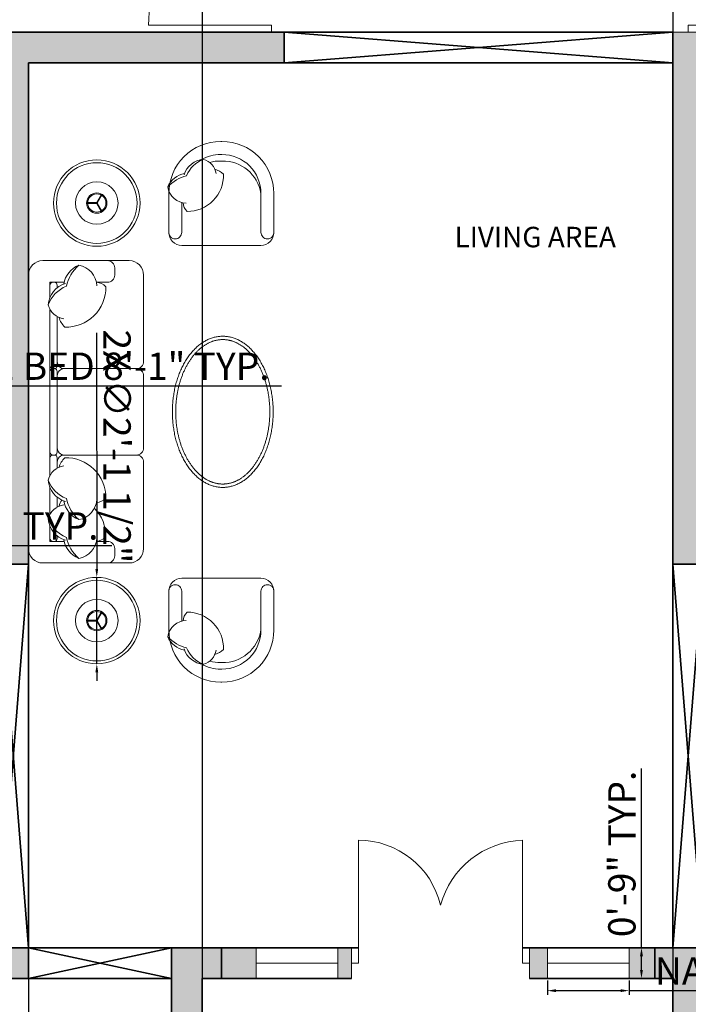
# Model space of a CAD drawing. Units: inches. Extents: x 2257 to 3678, y 834 to 1975.
# Tile 3 of 16: x 2500 to 2696, y 1155 to 1444. Entities that reach past the tile are written whole.
import ezdxf

# ---------------------------------------------------------------- set-up
doc = ezdxf.new("R2010")
doc.units = ezdxf.units.IN
for name, color, linetype, lineweight in [('A-ANNO-DIMS', 2, 'Continuous', 18), ('A-AREA-IDEN', 7, 'Continuous', 18), ('A-DOOR', 3, 'Continuous', 18), ('A-FURN', 8, 'Continuous', 18), ('A-GLAZ', 4, 'Continuous', 18), ('A-WALL', 7, 'Continuous', 35)]:
    doc.layers.add(name, color=color, linetype=linetype, lineweight=lineweight)
doc.layers.add('A-WALL-PATT', color=251, linetype='Continuous', lineweight=13, true_color=0x636466)
doc.styles.get("Standard").update_dxf_attribs({"font": 'arial.ttf'})
doc.dimstyles.new('ISO-25', dxfattribs={"dimtxt": 8, "dimasz": 2.5, "dimexe": 1.25, "dimexo": 0.625, "dimtad": 1, "dimdec": 0, "dimlunit": 3, "dimtxsty": 'Standard', "dimcen": 2.5, "dimadec": 0, "dimazin": 0, "dimtfac": 1, "dimtdec": 0, "dimtmove": 0, "dimatfit": 3, "dimfxl": 1, "dimarcsym": 0})

# ---------------------------------------------------------------- blocks, each defined once
blk = doc.blocks.new('TABLE-END-ROUND')
at = {"ltscale": 0.03}
for p, q in [((12.55, 12.73), (14.04, 15.31)), ((12.78, 12.6), (14.27, 15.18)), ((12.67, 12.8), (9.69, 12.8)), ((12.67, 12.53), (9.69, 12.53)), ((12.55, 12.6), (14.04, 10.02)), ((12.78, 12.73), (14.27, 10.15))]:
    blk.add_line(p, q, dxfattribs=at)
for radius in [12.67, 6.23, 2.98, 2.67]:
    blk.add_circle((12.67, 12.67), radius, dxfattribs=at)
blk.add_circle((12.67, 12.67), 11.82)
blk = doc.blocks.new('WIN-24')
for p, q in [((0, 9), (0, 0)), ((24, 4.5), (24, 9)), ((24, 9), (24, 0)), ((0, 0), (0, 4.5)), ((0, 4.5), (24, 4.5))]:
    blk.add_line(p, q)
blk = doc.blocks.new('DOOR-BEDROOM-REAR')
for p, q in [((36, 45), (36, 43)), ((36, 2), (0, 2)), ((36, 0), (36, 2))]:
    blk.add_line(p, q)
blk.add_arc((41.35, 2), 41.35, 97.4306, 180)
blk = doc.blocks.new('DOOR-KITCHEN')
for p, q in [((0, 45), (9, 45)), ((4.5, 45), (4.5, 43)), ((9, 45), (4.5, 45)), ((4.5, 0), (4.5, 2)), ((4.5, 2), (40.5, 2)), ((9, 0), (0, 0))]:
    blk.add_line(p, q)
blk.add_arc((4.5, 6.7), 36.3, 352.5694, 90)
blk = doc.blocks.new('DOOR-LOBBY-PAIR')
for p, q in [((2, 4.5), (2, 40.5)), ((50.14, 4.5), (50.14, 40.5)), ((0, 0), (0, 9)), ((0, 9), (0, 4.5)), ((52.14, 9), (52.14, 0)), ((0, 4.5), (2, 4.5)), ((52.14, 4.5), (50.14, 4.5)), ((52.14, 0), (52.14, 4.5))]:
    blk.add_line(p, q)
for centre, radius, start, end in [((2, 15.75), 24.75, 13.3945, 90), ((50.98, 14.71), 25.8, 91.8668, 164.7875)]:
    blk.add_arc(centre, radius, start, end)
blk = doc.blocks.new('*D48')
at = {"layer": 'A-ANNO-DIMS', "color": 0, "lineweight": -2, "transparency": 16777216}
for p, q in [((2351.99, 1350.73), (2351.99, 1335.55)), ((2448.99, 1350.73), (2448.99, 1335.55)), ((2354.49, 1336.8), (2446.49, 1336.8)), ((2448.99, 1336.8), (2576.25, 1336.8))]:
    blk.add_line(p, q, dxfattribs=at)
at = {"layer": 'A-ANNO-DIMS', "color": 0, "transparency": 16777216}
for points in [[(2354.49, 1337.22), (2354.49, 1336.39), (2351.99, 1336.8)], [(2446.49, 1337.22), (2446.49, 1336.39), (2448.99, 1336.8)]]:
    blk.add_solid(points, dxfattribs=at)
at = {"layer": 'Defpoints', "color": 0, "transparency": 16777216}
for p in [(2351.99, 1351.35), (2448.99, 1351.35), (2448.99, 1336.8)]:
    blk.add_point(p, dxfattribs=at)
at = {"layer": 'A-ANNO-DIMS', "color": 0, "transparency": 16777216, "insert": (2513.87, 1341.57), "char_height": 8, "attachment_point": 5}
blk.add_mtext('DOUBLE BED 8\'-1" TYP.', dxfattribs=at)
blk = doc.blocks.new('*D60')
at = {"layer": 'A-ANNO-DIMS', "color": 0, "lineweight": -2, "transparency": 16777216}
for p, q in [((2654.22, 1162.45), (2654.22, 1158.23)), ((2678.22, 1162.45), (2678.22, 1158.23)), ((2656.72, 1159.48), (2675.72, 1159.48)), ((2678.22, 1159.48), (2836.5, 1159.48))]:
    blk.add_line(p, q, dxfattribs=at)
at = {"layer": 'A-ANNO-DIMS', "color": 0, "transparency": 16777216}
for points in [[(2656.72, 1159.89), (2656.72, 1159.06), (2654.22, 1159.48)], [(2675.72, 1159.89), (2675.72, 1159.06), (2678.22, 1159.48)]]:
    blk.add_solid(points, dxfattribs=at)
at = {"layer": 'Defpoints', "color": 0, "transparency": 16777216}
for p in [(2654.22, 1163.08), (2678.22, 1163.08), (2678.22, 1159.48)]:
    blk.add_point(p, dxfattribs=at)
at = {"layer": 'A-ANNO-DIMS', "color": 0, "transparency": 16777216, "insert": (2758.61, 1164.24), "char_height": 8, "attachment_point": 5}
blk.add_mtext('NARROW WINDOW 2\'-0" TYP.', dxfattribs=at)
blk = doc.blocks.new('*D61')
at = {"layer": 'A-ANNO-DIMS', "color": 0, "lineweight": -2, "transparency": 16777216}
for p, q in [((2681.82, 1172.08), (2681.82, 1224.59)), ((2678.85, 1172.08), (2683.07, 1172.08)), ((2681.82, 1165.58), (2681.82, 1169.58)), ((2678.85, 1163.08), (2683.07, 1163.08))]:
    blk.add_line(p, q, dxfattribs=at)
at = {"layer": 'A-ANNO-DIMS', "color": 0, "transparency": 16777216}
for points in [[(2681.4, 1169.58), (2682.24, 1169.58), (2681.82, 1172.08)], [(2681.4, 1165.58), (2682.24, 1165.58), (2681.82, 1163.08)]]:
    blk.add_solid(points, dxfattribs=at)
at = {"layer": 'Defpoints', "color": 0, "transparency": 16777216}
for p in [(2678.22, 1172.08), (2681.82, 1172.08), (2678.22, 1163.08)]:
    blk.add_point(p, dxfattribs=at)
at = {"layer": 'A-ANNO-DIMS', "color": 0, "transparency": 16777216, "insert": (2677.11, 1199.58), "char_height": 8, "attachment_point": 5, "rotation": 90}
blk.add_mtext('0\'-9" TYP.', dxfattribs=at)
blk = doc.blocks.new('*D80')
at = {"layer": 'A-ANNO-DIMS', "color": 0, "lineweight": -2, "transparency": 16777216}
for p, q in [((2372.21, 1285.2), (2372.21, 1291.23)), ((2408.21, 1285.2), (2408.21, 1291.23)), ((2374.71, 1289.98), (2405.71, 1289.98)), ((2408.21, 1289.98), (2526.51, 1289.98))]:
    blk.add_line(p, q, dxfattribs=at)
at = {"layer": 'A-ANNO-DIMS', "color": 0, "transparency": 16777216}
for points in [[(2374.71, 1290.39), (2374.71, 1289.56), (2372.21, 1289.98)], [(2405.71, 1290.39), (2405.71, 1289.56), (2408.21, 1289.98)]]:
    blk.add_solid(points, dxfattribs=at)
at = {"layer": 'Defpoints', "color": 0, "transparency": 16777216}
for p in [(2408.21, 1289.98), (2372.21, 1284.58), (2408.21, 1284.58)]:
    blk.add_point(p, dxfattribs=at)
at = {"layer": 'A-ANNO-DIMS', "color": 0, "transparency": 16777216, "insert": (2468.61, 1294.74), "char_height": 8, "attachment_point": 5}
blk.add_mtext('SIDE DOOR 3\'-0" TYP.', dxfattribs=at)
blk = doc.blocks.new('*D96')
at = {"layer": 'A-ANNO-DIMS', "color": 0, "lineweight": -2, "transparency": 16777216}
for p, q in [((2337.05, 1283.95), (2337.05, 894.3)), ((2883.34, 1168.45), (2883.34, 894.3)), ((2339.55, 895.55), (2880.84, 895.55))]:
    blk.add_line(p, q, dxfattribs=at)
at = {"layer": 'A-ANNO-DIMS', "color": 0, "transparency": 16777216}
for points in [[(2339.55, 895.97), (2339.55, 895.14), (2337.05, 895.55)], [(2880.84, 895.97), (2880.84, 895.14), (2883.34, 895.55)]]:
    blk.add_solid(points, dxfattribs=at)
at = {"layer": 'Defpoints', "color": 0, "transparency": 16777216}
for p in [(2337.05, 1284.58), (2883.34, 1169.08), (2883.34, 895.55)]:
    blk.add_point(p, dxfattribs=at)
at = {"layer": 'A-ANNO-DIMS', "color": 0, "transparency": 16777216, "insert": (2610.2, 900.31), "char_height": 8, "attachment_point": 5}
blk.add_mtext('45\'-6 1/2"', dxfattribs=at)
blk = doc.blocks.new('*D106')
at = {"layer": 'A-ANNO-DIMS', "color": 0, "lineweight": -2, "transparency": 16777216}
for p, q in [((2553.05, 1583.95), (2553.05, 894.3)), ((2691.05, 1583.95), (2691.05, 894.3)), ((2555.55, 895.55), (2688.55, 895.55))]:
    blk.add_line(p, q, dxfattribs=at)
at = {"layer": 'A-ANNO-DIMS', "color": 0, "transparency": 16777216}
for points in [[(2555.55, 895.97), (2555.55, 895.14), (2553.05, 895.55)], [(2688.55, 895.97), (2688.55, 895.14), (2691.05, 895.55)]]:
    blk.add_solid(points, dxfattribs=at)
at = {"layer": 'Defpoints', "color": 0, "transparency": 16777216}
for p in [(2553.05, 1584.58), (2691.05, 1584.58), (2691.05, 895.55)]:
    blk.add_point(p, dxfattribs=at)
at = {"layer": 'A-ANNO-DIMS', "color": 0, "transparency": 16777216, "insert": (2622.05, 900.26), "char_height": 8, "attachment_point": 5}
blk.add_mtext('11\'-6"', dxfattribs=at)
blk = doc.blocks.new('*D107')
at = {"layer": 'A-ANNO-DIMS', "color": 0, "lineweight": -2, "transparency": 16777216}
for p, q in [((2502.05, 1430.95), (2502.05, 894.3)), ((2691.05, 1430.95), (2691.05, 894.3)), ((2504.55, 895.55), (2688.55, 895.55))]:
    blk.add_line(p, q, dxfattribs=at)
at = {"layer": 'A-ANNO-DIMS', "color": 0, "transparency": 16777216}
for points in [[(2504.55, 895.97), (2504.55, 895.14), (2502.05, 895.55)], [(2688.55, 895.97), (2688.55, 895.14), (2691.05, 895.55)]]:
    blk.add_solid(points, dxfattribs=at)
at = {"layer": 'Defpoints', "color": 0, "transparency": 16777216}
for p in [(2502.05, 1431.58), (2691.05, 1431.58), (2691.05, 895.55)]:
    blk.add_point(p, dxfattribs=at)
at = {"layer": 'A-ANNO-DIMS', "color": 0, "transparency": 16777216, "insert": (2596.55, 900.26), "char_height": 8, "attachment_point": 5}
blk.add_mtext('15\'-9"', dxfattribs=at)
blk = doc.blocks.new('*D151')
at = {"layer": 'A-ANNO-DIMS', "color": 0, "lineweight": -2, "transparency": 16777216}
for p, q in [((2522.07, 1352.44), (2522.1, 1283.18)), ((2522.11, 1255.35), (2522.1, 1280.68)), ((2522.11, 1252.85), (2522.11, 1250.35))]:
    blk.add_line(p, q, dxfattribs=at)
at = {"layer": 'A-ANNO-DIMS', "color": 0, "transparency": 16777216}
for points in [[(2522.52, 1283.18), (2521.68, 1283.18), (2522.1, 1280.68)], [(2522.53, 1252.85), (2521.7, 1252.84), (2522.11, 1255.35)]]:
    blk.add_solid(points, dxfattribs=at)
at = {"layer": 'Defpoints', "color": 0, "transparency": 16777216}
for p in [(2522.1, 1280.68), (2522.11, 1255.35)]:
    blk.add_point(p, dxfattribs=at)
at = {"layer": 'A-ANNO-DIMS', "color": 0, "transparency": 16777216, "insert": (2527.02, 1319.06), "char_height": 8, "attachment_point": 5, "rotation": 270.0256}
blk.add_mtext('2X ∅2\'-1 1/2"', dxfattribs=at)

msp = doc.modelspace()

# ---------------------------------------------------------------- hatches: boundary and pattern name
at = {"layer": 'A-WALL-PATT'}
h = msp.add_hatch(color=256, dxfattribs=at)
h.dxf.hatch_style = 1
h.paths.add_polyline_path([(2736.02, 1589.08), (2736.02, 1593.58), (2691.05, 1593.58), (2648.2, 1593.58), (2648.2, 1584.58), (2691.05, 1584.58), (2691.05, 1485.58), (2700.05, 1485.58), (2700.05, 1584.58), (2736.02, 1584.58)])
h.paths.add_polyline_path([(2835.05, 1593.58), (2796.02, 1593.58), (2796.02, 1584.58), (2826.05, 1584.58), (2826.05, 1440.58), (2835.05, 1440.58)])
h.paths.add_polyline_path([(2865.05, 1440.58), (2826.05, 1440.58), (2700.05, 1440.58), (2691.05, 1440.58), (2691.05, 1431.58), (2691.05, 1284.58), (2700.05, 1284.58), (2700.05, 1431.58), (2826.05, 1431.58), (2856.05, 1431.58), (2856.05, 1395.2), (2865.05, 1395.2), (2865.05, 1431.58)])
h.paths.add_polyline_path([(2865.05, 1335.2), (2856.05, 1335.2), (2856.05, 1293.58), (2741.94, 1293.58), (2741.94, 1289.08), (2741.94, 1284.58), (2865.05, 1284.58)], flags=17)
h.paths.add_polyline_path([(2865.05, 1172.08), (2856.05, 1172.08), (2741.94, 1172.08), (2741.94, 1163.08), (2856.05, 1163.08), (2856.05, 1133.53), (2865.05, 1133.53)])
h.paths.add_polyline_path([(2865.05, 1073.53), (2856.05, 1073.53), (2856.05, 1019.08), (2795.28, 1019.08), (2795.28, 1010.08), (2865.05, 1010.08)])
h.paths.add_polyline_path([(2735.28, 1014.58), (2735.28, 1019.08), (2700.05, 1019.08), (2700.05, 1026.35), (2695.55, 1026.35), (2691.05, 1026.35), (2691.05, 1010.08), (2735.28, 1010.08)])
h.paths.add_polyline_path([(2700.05, 1163.08), (2700.05, 1172.08), (2691.05, 1172.08), (2685.7, 1172.08), (2685.7, 1163.08), (2691.05, 1163.08), (2691.05, 1058.19), (2700.05, 1058.19)])
h.paths.add_polyline_path([(2707.1, 1172.08), (2700.05, 1172.08), (2700.05, 1163.08), (2707.1, 1163.08)])
h.paths.add_polyline_path([(2685.7, 1172.08), (2678.22, 1172.08), (2678.22, 1163.08), (2685.7, 1163.08)])
h.paths.add_polyline_path([(2654.22, 1172.08), (2648.96, 1172.08), (2648.96, 1163.08), (2654.22, 1163.08), (2654.22, 1167.58)])
h.paths.add_polyline_path([(2553.05, 1163.08), (2558.66, 1163.08), (2558.66, 1172.08), (2544.05, 1172.08), (2544.05, 1163.08), (2544.05, 1058.19), (2553.05, 1058.19)])
h.paths.add_polyline_path([(2568.8, 1167.58), (2568.8, 1172.08), (2558.66, 1172.08), (2558.66, 1163.08), (2568.8, 1163.08)])
h.paths.add_polyline_path([(2596.82, 1172.08), (2592.8, 1172.08), (2592.8, 1163.08), (2596.82, 1163.08)])
h.paths.add_polyline_path([(2553.05, 1019.08), (2553.05, 1026.35), (2548.55, 1026.35), (2544.05, 1026.35), (2544.05, 1019.08), (2476.8, 1019.08), (2476.8, 1010.08), (2553.05, 1010.08)])
h.paths.add_polyline_path([(2376.05, 1163.08), (2502.05, 1163.08), (2502.05, 1172.08), (2446.55, 1172.08), (2446.55, 1195.52), (2446.55, 1215.32), (2442.05, 1215.32), (2442.05, 1195.52), (2442.05, 1172.08), (2412.05, 1172.08), (2412.05, 1167.58), (2376.05, 1167.58), (2376.05, 1172.08), (2376.05, 1201.28), (2367.05, 1201.28), (2367.05, 1172.08), (2367.05, 1123.86), (2376.05, 1123.86)])
h.paths.add_polyline_path([(2577.05, 1440.58), (2376.05, 1440.58), (2376.05, 1485.89), (2367.05, 1485.89), (2367.05, 1440.58), (2337.05, 1440.58), (2337.05, 1403.59), (2346.05, 1403.59), (2346.05, 1431.58), (2493.05, 1431.58), (2493.05, 1293.58), (2484.41, 1293.58), (2484.41, 1284.58), (2502.05, 1284.58), (2502.05, 1431.58), (2577.05, 1431.58)])
h.paths.add_polyline_path([(2346.05, 1343.59), (2337.05, 1343.59), (2337.05, 1284.58), (2448.12, 1284.58), (2448.12, 1289.08), (2448.12, 1293.58), (2346.05, 1293.58)], flags=17)
h.paths.add_polyline_path([(2376.05, 1244.08), (2446.55, 1244.08), (2446.55, 1248.58), (2367.05, 1248.58), (2367.05, 1225.28), (2375.64, 1225.28), (2375.64, 1228.02), (2376.05, 1228.02)])
h.paths.add_polyline_path([(2588.2, 1589.08), (2588.2, 1593.58), (2468.1, 1593.58), (2468.1, 1584.58), (2544.05, 1584.58), (2544.05, 1541.08), (2568.05, 1541.08), (2568.05, 1490.08), (2544.05, 1490.08), (2544.05, 1485.58), (2577.05, 1485.58), (2577.05, 1545.58), (2553.05, 1545.58), (2553.05, 1584.58), (2588.2, 1584.58)])
h.paths.add_polyline_path([(2376.05, 1584.58), (2408.1, 1584.58), (2408.1, 1589.08), (2408.1, 1593.58), (2367.05, 1593.58), (2367.05, 1545.89), (2376.05, 1545.89)])
h.paths.add_polyline_path([(2376.05, 1063.86), (2367.05, 1063.86), (2367.05, 1019.08), (2367.05, 1010.08), (2416.8, 1010.08), (2416.8, 1014.58), (2416.8, 1019.08), (2376.05, 1019.08)])

# ---------------------------------------------------------------- linework, layer by layer
at = {"layer": 'A-FURN', "ltscale": 0.03}
for points in [[(2558.63, 1378.04), (2570.24, 1378.04, 0.414214), (2574.04, 1381.85), (2574.04, 1393.27, 0.414214), (2558.82, 1408.49), (2558.63, 1408.49), (2558.44, 1408.49, 0.414214), (2543.21, 1393.27), (2543.21, 1381.85, 0.414214), (2547.02, 1378.04), (2558.63, 1378.04)], [(2558.63, 1280.42), (2570.24, 1280.42, -0.414214), (2574.04, 1276.61), (2574.04, 1265.19, -0.414214), (2558.82, 1249.97), (2558.63, 1249.97), (2558.44, 1249.97, -0.414214), (2543.21, 1265.19), (2543.21, 1276.61, -0.414214), (2547.02, 1280.42), (2558.63, 1280.42)]]:
    msp.add_lwpolyline(points, format="xyb", dxfattribs=at)
at = {"layer": 'A-FURN'}
for points in [[(2552.77, 1403.18, -0.130591), (2558.44, 1404.69), (2558.63, 1404.69)], [(2570.24, 1393.27, 0.414214), (2558.82, 1404.69), (2558.63, 1404.69)], [(2542.9, 1395.19, -0.14773), (2548.46, 1398.46, -0.213343), (2553.37, 1403.26, -0.178662)], [(2547.69, 1398.72, -0.306663), (2553.37, 1403.26, -0.30633), (2557.08, 1399.11, 0.872847)], [(2555.19, 1402.37, -0.072384), (2558.44, 1402.78), (2558.63, 1402.78)], [(2570.24, 1393.27, 0.372719), (2558.82, 1402.78), (2558.63, 1402.78)], [(2548.35, 1390.39, -0.356772), (2542.9, 1395.19, -0.249542), (2547.84, 1399.14, 9.61688)], [(2547.39, 1390.51, 0.165541), (2548.57, 1387.99, 0.425989), (2559.26, 1398.9, 0.121523), (2556.72, 1400.4, -7.115464)], [(2570.24, 1393.27), (2570.24, 1381.85, 0.414214), (2572.14, 1379.94), (2572.14, 1379.94, 0.414214), (2574.04, 1381.85)], [(2547.02, 1390.6), (2547.02, 1381.85, -0.414214), (2545.11, 1379.94), (2545.11, 1379.94, -0.414214), (2543.21, 1381.85)], [(2516.81, 1372.22, 0.14773), (2513.18, 1366.05, 0.213343), (2507.86, 1360.6, 0.178662)], [(2522.13, 1366.17, 0.356772), (2516.81, 1372.22, 0.249542), (2512.42, 1366.74, -9.61688)], [(2525.27, 1373.56, -0.414214), (2527.38, 1371.45), (2527.38, 1369.34, -0.414214), (2525.27, 1367.23), (2522, 1367.23)], [(2512.89, 1366.9, 0.306663), (2507.86, 1360.6, 0.30633), (2512.45, 1356.49, -0.872847)], [(2510.5, 1365.62), (2510.5, 1366.38, 0.414214), (2509.65, 1367.23), (2509.23, 1367.23, 0.414214), (2508.38, 1366.38)], [(2508.38, 1366.38), (2508.38, 1362.79, 0.414214)], [(2522, 1367.23, -0.165541), (2524.79, 1365.93, -0.425989), (2512.7, 1354.07, -0.121523), (2511.03, 1356.89, 7.115464)], [(2508.38, 1359.28), (2508.38, 1342.74, 0.414214), (2509.23, 1341.9), (2509.65, 1341.9, 0.414214), (2510.5, 1342.74), (2510.5, 1357.15, 0.414214)], [(2510.5, 1344.01, 0.414214), (2512.61, 1341.9), (2533.72, 1341.9, 0.414214)], [(2510.5, 1339.79, -0.414214), (2512.61, 1341.9)], [(2510.5, 1318.68, 0.414214), (2512.61, 1316.56)], [(2508.38, 1310.56), (2508.38, 1315.72, -0.414214), (2509.23, 1316.56), (2509.65, 1316.56, -0.414214), (2510.5, 1315.72), (2510.5, 1312.68, -0.414214)], [(2510.5, 1314.45, -0.414214), (2512.61, 1316.56), (2533.72, 1316.56, -0.414214)], [(2522, 1302.6, 0.165541), (2524.79, 1303.91, 0.425989), (2512.7, 1315.76, 0.121523), (2511.03, 1312.95, -7.115464)], [(2512.89, 1302.93, -0.306663), (2507.86, 1309.23, -0.30633), (2512.45, 1313.34, 0.872847)], [(2516.81, 1297.61, -0.14773), (2513.18, 1303.78, -0.213343), (2507.86, 1309.23, -0.178662)], [(2508.38, 1299.19), (2508.38, 1307.05, -0.414214)], [(2510.5, 1304.22), (2510.5, 1301.31, -0.414214)], [(2511.85, 1303.35, 0.071865), (2511.03, 1301.58, -7.115464)], [(2522.13, 1303.66, -0.356772), (2516.81, 1297.61, -0.249542), (2512.42, 1303.1, 9.61688)], [(2512.89, 1291.56, -0.306663), (2507.86, 1297.86, -0.30633), (2512.45, 1301.97, 0.872847)], [(2522, 1291.23, 0.165541), (2524.79, 1292.53, 0.200231), (2521.39, 1300.91, 0.121523)], [(2516.81, 1286.24, -0.14773), (2513.18, 1292.41, -0.213343), (2507.86, 1297.86, -0.178662)], [(2508.38, 1295.67), (2508.38, 1291.23), (2512.53, 1291.23, -0.414214)], [(2508.38, 1292.08), (2508.38, 1295.67, -0.414214)], [(2510.5, 1292.84), (2510.5, 1292.08, -0.414214), (2509.65, 1291.23), (2509.23, 1291.23, -0.414214), (2508.38, 1292.08)], [(2522.13, 1292.29, -0.356772), (2516.81, 1286.24, -0.249542), (2512.42, 1291.72, 9.61688)], [(2522, 1291.23), (2525.27, 1291.23, -0.414214), (2527.38, 1289.12), (2527.38, 1287.01, -0.414214), (2525.27, 1284.9)], [(2547.02, 1267.86), (2547.02, 1276.61, 0.414214), (2545.11, 1278.52), (2545.11, 1278.52, 0.414214), (2543.21, 1276.61)], [(2570.24, 1265.19), (2570.24, 1276.61, -0.414214), (2572.14, 1278.52), (2572.14, 1278.52, -0.414214), (2574.04, 1276.61)], [(2548.35, 1268.07, 0.356772), (2542.9, 1263.27, 0.249542), (2547.84, 1259.32, -9.61688)], [(2547.39, 1267.95, -0.165541), (2548.57, 1270.47, -0.425989), (2559.26, 1259.57, -0.121523), (2556.72, 1258.06, 7.115464)], [(2570.24, 1265.19, -0.372719), (2558.82, 1255.68), (2558.63, 1255.68)], [(2570.24, 1265.19, -0.414214), (2558.82, 1253.77), (2558.63, 1253.77)], [(2542.9, 1263.27, 0.14773), (2548.46, 1260, 0.213343), (2553.37, 1255.2, 0.178662)], [(2547.69, 1259.74, 0.306663), (2553.37, 1255.2, 0.30633), (2557.08, 1259.35, -0.872847)], [(2555.19, 1256.09, 0.072384), (2558.44, 1255.68), (2558.63, 1255.68)], [(2552.77, 1255.28, 0.130591), (2558.44, 1253.77), (2558.63, 1253.77)]]:
    msp.add_lwpolyline(points, format="xyb", dxfattribs=at)
at = {"layer": 'A-FURN', "ltscale": 0.03}
msp.add_lwpolyline([(2531.61, 1373.56, -0.414214), (2535.83, 1369.34), (2535.83, 1344.01, -0.414214), (2533.72, 1341.9, -0.414214), (2535.83, 1339.79), (2535.83, 1318.68, -0.414214), (2533.72, 1316.56, -0.414214), (2535.83, 1314.45), (2535.83, 1289.12, -0.414214), (2531.61, 1284.9), (2506.27, 1284.9, -0.414214), (2502.05, 1289.12), (2502.05, 1369.34, -0.414214), (2506.27, 1373.56)], format="xyb", close=True, dxfattribs=at)
at = {"layer": 'A-FURN'}
for points in [[(2512.53, 1367.23), (2508.38, 1367.23), (2508.38, 1362.79)], [(2508.38, 1359.28), (2508.38, 1310.56)], [(2508.38, 1307.05), (2508.38, 1299.19)]]:
    msp.add_lwpolyline(points, dxfattribs=at)
msp.add_lwpolyline([(2508.38, 1317.41), (2508.38, 1341.05, -0.414214), (2509.23, 1341.9), (2509.65, 1341.9, -0.414214), (2510.5, 1341.05), (2510.5, 1317.41, -0.414214), (2509.65, 1316.56), (2509.23, 1316.56, -0.414214)], format="xyb", close=True, dxfattribs=at)
at = {"layer": 'A-FURN', "ltscale": 0.03}
msp.add_polyline3d([(2559.05, 1351.4, 0), (2558.77, 1351.39, 0), (2558.49, 1351.38, 0), (2558.21, 1351.36, 0), (2557.93, 1351.33, 0), (2557.65, 1351.3, 0), (2557.37, 1351.25, 0), (2557.1, 1351.2, 0), (2556.82, 1351.14, 0), (2556.54, 1351.08, 0), (2556.27, 1351, 0), (2555.99, 1350.92, 0), (2555.72, 1350.83, 0), (2555.45, 1350.73, 0), (2555.18, 1350.62, 0), (2554.91, 1350.51, 0), (2554.64, 1350.39, 0), (2554.38, 1350.26, 0), (2554.11, 1350.12, 0), (2553.85, 1349.98, 0), (2553.59, 1349.83, 0), (2553.33, 1349.67, 0), (2553.07, 1349.5, 0), (2552.82, 1349.33, 0), (2552.57, 1349.15, 0), (2552.31, 1348.96, 0), (2552.07, 1348.77, 0), (2551.82, 1348.57, 0), (2551.58, 1348.36, 0), (2551.34, 1348.14, 0), (2551.1, 1347.92, 0), (2550.87, 1347.69, 0), (2550.64, 1347.45, 0), (2550.41, 1347.21, 0), (2550.18, 1346.96, 0), (2549.96, 1346.71, 0), (2549.74, 1346.45, 0), (2549.53, 1346.18, 0), (2549.31, 1345.91, 0), (2549.11, 1345.63, 0), (2548.9, 1345.34, 0), (2548.7, 1345.05, 0), (2548.5, 1344.76, 0), (2548.31, 1344.45, 0), (2548.12, 1344.15, 0), (2547.93, 1343.83, 0), (2547.75, 1343.51, 0), (2547.57, 1343.19, 0), (2547.4, 1342.86, 0), (2547.23, 1342.53, 0), (2547.06, 1342.19, 0), (2546.9, 1341.85, 0), (2546.74, 1341.5, 0), (2546.59, 1341.15, 0), (2546.44, 1340.79, 0), (2546.3, 1340.43, 0), (2546.16, 1340.07, 0), (2546.02, 1339.7, 0), (2545.89, 1339.33, 0), (2545.77, 1338.96, 0), (2545.65, 1338.58, 0), (2545.53, 1338.2, 0), (2545.42, 1337.81, 0), (2545.32, 1337.42, 0), (2545.22, 1337.03, 0), (2545.12, 1336.64, 0), (2545.03, 1336.24, 0), (2544.94, 1335.84, 0), (2544.86, 1335.44, 0), (2544.79, 1335.04, 0), (2544.72, 1334.63, 0), (2544.65, 1334.22, 0), (2544.59, 1333.81, 0), (2544.54, 1333.4, 0), (2544.49, 1332.99, 0), (2544.44, 1332.57, 0), (2544.4, 1332.16, 0), (2544.37, 1331.74, 0), (2544.34, 1331.33, 0), (2544.31, 1330.91, 0), (2544.3, 1330.49, 0), (2544.28, 1330.07, 0), (2544.27, 1329.65, 0), (2544.27, 1329.23, 0), (2544.27, 1328.81, 0), (2544.28, 1328.39, 0), (2544.3, 1327.97, 0), (2544.31, 1327.55, 0), (2544.34, 1327.14, 0), (2544.37, 1326.72, 0), (2544.4, 1326.3, 0), (2544.44, 1325.89, 0), (2544.49, 1325.47, 0), (2544.54, 1325.06, 0), (2544.59, 1324.65, 0), (2544.65, 1324.24, 0), (2544.72, 1323.83, 0), (2544.79, 1323.43, 0), (2544.86, 1323.02, 0), (2544.94, 1322.62, 0), (2545.03, 1322.22, 0), (2545.12, 1321.83, 0), (2545.22, 1321.43, 0), (2545.32, 1321.04, 0), (2545.42, 1320.65, 0), (2545.53, 1320.27, 0), (2545.65, 1319.88, 0), (2545.77, 1319.51, 0), (2545.89, 1319.13, 0), (2546.02, 1318.76, 0), (2546.16, 1318.39, 0), (2546.3, 1318.03, 0), (2546.44, 1317.67, 0), (2546.59, 1317.31, 0), (2546.74, 1316.96, 0), (2546.9, 1316.61, 0), (2547.06, 1316.27, 0), (2547.23, 1315.93, 0), (2547.4, 1315.6, 0), (2547.57, 1315.27, 0), (2547.75, 1314.95, 0), (2547.93, 1314.63, 0), (2548.12, 1314.32, 0), (2548.31, 1314.01, 0), (2548.5, 1313.71, 0), (2548.7, 1313.41, 0), (2548.9, 1313.12, 0), (2549.11, 1312.83, 0), (2549.31, 1312.55, 0), (2549.53, 1312.28, 0), (2549.74, 1312.01, 0), (2549.96, 1311.75, 0), (2550.18, 1311.5, 0), (2550.41, 1311.25, 0), (2550.64, 1311.01, 0), (2550.87, 1310.77, 0), (2551.1, 1310.54, 0), (2551.34, 1310.32, 0), (2551.58, 1310.11, 0), (2551.82, 1309.9, 0), (2552.07, 1309.69, 0), (2552.31, 1309.5, 0), (2552.57, 1309.31, 0), (2552.82, 1309.13, 0), (2553.07, 1308.96, 0), (2553.33, 1308.79, 0), (2553.59, 1308.63, 0), (2553.85, 1308.48, 0), (2554.11, 1308.34, 0), (2554.38, 1308.2, 0), (2554.64, 1308.07, 0), (2554.91, 1307.95, 0), (2555.18, 1307.84, 0), (2555.45, 1307.73, 0), (2555.72, 1307.63, 0), (2555.99, 1307.54, 0), (2556.27, 1307.46, 0), (2556.54, 1307.39, 0), (2556.82, 1307.32, 0), (2557.1, 1307.26, 0), (2557.37, 1307.21, 0), (2557.65, 1307.16, 0), (2557.93, 1307.13, 0), (2558.21, 1307.1, 0), (2558.49, 1307.08, 0), (2558.77, 1307.07, 0), (2559.05, 1307.07, 0), (2559.33, 1307.07, 0), (2559.61, 1307.08, 0), (2559.89, 1307.1, 0), (2560.17, 1307.13, 0), (2560.44, 1307.16, 0), (2560.72, 1307.21, 0), (2561, 1307.26, 0), (2561.28, 1307.32, 0), (2561.55, 1307.39, 0), (2561.83, 1307.46, 0), (2562.1, 1307.54, 0), (2562.38, 1307.63, 0), (2562.65, 1307.73, 0), (2562.92, 1307.84, 0), (2563.19, 1307.95, 0), (2563.46, 1308.07, 0), (2563.72, 1308.2, 0), (2563.99, 1308.34, 0), (2564.25, 1308.48, 0), (2564.51, 1308.63, 0), (2564.77, 1308.79, 0), (2565.02, 1308.96, 0), (2565.28, 1309.13, 0), (2565.53, 1309.31, 0), (2565.78, 1309.5, 0), (2566.03, 1309.69, 0), (2566.28, 1309.9, 0), (2566.52, 1310.11, 0), (2566.76, 1310.32, 0), (2566.99, 1310.54, 0), (2567.23, 1310.77, 0), (2567.46, 1311.01, 0), (2567.69, 1311.25, 0), (2567.91, 1311.5, 0), (2568.14, 1311.75, 0), (2568.36, 1312.01, 0), (2568.57, 1312.28, 0), (2568.78, 1312.55, 0), (2568.99, 1312.83, 0), (2569.2, 1313.12, 0), (2569.4, 1313.41, 0), (2569.6, 1313.71, 0), (2569.79, 1314.01, 0), (2569.98, 1314.32, 0), (2570.17, 1314.63, 0), (2570.35, 1314.95, 0), (2570.53, 1315.27, 0), (2570.7, 1315.6, 0), (2570.87, 1315.93, 0), (2571.04, 1316.27, 0), (2571.2, 1316.61, 0), (2571.35, 1316.96, 0), (2571.51, 1317.31, 0), (2571.66, 1317.67, 0), (2571.8, 1318.03, 0), (2571.94, 1318.39, 0), (2572.07, 1318.76, 0), (2572.2, 1319.13, 0), (2572.33, 1319.51, 0), (2572.45, 1319.88, 0), (2572.56, 1320.27, 0), (2572.67, 1320.65, 0), (2572.78, 1321.04, 0), (2572.88, 1321.43, 0), (2572.98, 1321.83, 0), (2573.07, 1322.22, 0), (2573.15, 1322.62, 0), (2573.23, 1323.02, 0), (2573.31, 1323.43, 0), (2573.38, 1323.83, 0), (2573.45, 1324.24, 0), (2573.51, 1324.65, 0), (2573.56, 1325.06, 0), (2573.61, 1325.47, 0), (2573.66, 1325.89, 0), (2573.7, 1326.3, 0), (2573.73, 1326.72, 0), (2573.76, 1327.14, 0), (2573.78, 1327.55, 0), (2573.8, 1327.97, 0), (2573.82, 1328.39, 0), (2573.82, 1328.81, 0), (2573.83, 1329.23, 0), (2573.82, 1329.65, 0), (2573.82, 1330.07, 0), (2573.8, 1330.49, 0), (2573.78, 1330.91, 0), (2573.76, 1331.33, 0), (2573.73, 1331.74, 0), (2573.7, 1332.16, 0), (2573.66, 1332.57, 0), (2573.61, 1332.99, 0), (2573.56, 1333.4, 0), (2573.51, 1333.81, 0), (2573.45, 1334.22, 0), (2573.38, 1334.63, 0), (2573.31, 1335.04, 0), (2573.23, 1335.44, 0), (2573.15, 1335.84, 0), (2573.07, 1336.24, 0), (2572.98, 1336.64, 0), (2572.88, 1337.03, 0), (2572.78, 1337.42, 0), (2572.67, 1337.81, 0), (2572.56, 1338.2, 0), (2572.45, 1338.58, 0), (2572.33, 1338.96, 0), (2572.2, 1339.33, 0), (2572.07, 1339.7, 0), (2571.94, 1340.07, 0), (2571.8, 1340.43, 0), (2571.66, 1340.79, 0), (2571.51, 1341.15, 0), (2571.35, 1341.5, 0), (2571.2, 1341.85, 0), (2571.04, 1342.19, 0), (2570.87, 1342.53, 0), (2570.7, 1342.86, 0), (2570.53, 1343.19, 0), (2570.35, 1343.51, 0), (2570.17, 1343.83, 0), (2569.98, 1344.15, 0), (2569.79, 1344.45, 0), (2569.6, 1344.76, 0), (2569.4, 1345.05, 0), (2569.2, 1345.34, 0), (2568.99, 1345.63, 0), (2568.78, 1345.91, 0), (2568.57, 1346.18, 0), (2568.36, 1346.45, 0), (2568.14, 1346.71, 0), (2567.91, 1346.96, 0), (2567.69, 1347.21, 0), (2567.46, 1347.45, 0), (2567.23, 1347.69, 0), (2566.99, 1347.92, 0), (2566.76, 1348.14, 0), (2566.52, 1348.36, 0), (2566.28, 1348.57, 0), (2566.03, 1348.77, 0), (2565.78, 1348.96, 0), (2565.53, 1349.15, 0), (2565.28, 1349.33, 0), (2565.02, 1349.5, 0), (2564.77, 1349.67, 0), (2564.51, 1349.83, 0), (2564.25, 1349.98, 0), (2563.99, 1350.12, 0), (2563.72, 1350.26, 0), (2563.46, 1350.39, 0), (2563.19, 1350.51, 0), (2562.92, 1350.62, 0), (2562.65, 1350.73, 0), (2562.38, 1350.83, 0), (2562.1, 1350.92, 0), (2561.83, 1351, 0), (2561.55, 1351.08, 0), (2561.28, 1351.14, 0), (2561, 1351.2, 0), (2560.72, 1351.25, 0), (2560.44, 1351.3, 0), (2560.17, 1351.33, 0), (2559.89, 1351.36, 0), (2559.61, 1351.38, 0), (2559.33, 1351.39, 0), (2559.05, 1351.4, 0)], dxfattribs=at)
at = {"layer": 'A-FURN'}
msp.add_polyline3d([(2559.05, 1350.41, 0), (2558.9, 1350.41, 0), (2558.75, 1350.41, 0), (2558.59, 1350.4, 0), (2558.44, 1350.39, 0), (2558.29, 1350.38, 0), (2558.13, 1350.36, 0), (2557.98, 1350.35, 0), (2557.82, 1350.33, 0), (2557.67, 1350.3, 0), (2557.51, 1350.28, 0), (2557.35, 1350.25, 0), (2557.19, 1350.22, 0), (2557.04, 1350.18, 0), (2556.88, 1350.14, 0), (2556.72, 1350.1, 0), (2556.56, 1350.06, 0), (2556.4, 1350.01, 0), (2556.24, 1349.96, 0), (2556.08, 1349.91, 0), (2555.92, 1349.85, 0), (2555.76, 1349.79, 0), (2555.6, 1349.73, 0), (2555.43, 1349.66, 0), (2555.27, 1349.59, 0), (2555.11, 1349.52, 0), (2554.95, 1349.44, 0), (2554.79, 1349.36, 0), (2554.62, 1349.28, 0), (2554.46, 1349.19, 0), (2554.3, 1349.1, 0), (2554.14, 1349.01, 0), (2553.98, 1348.91, 0), (2553.82, 1348.81, 0), (2553.66, 1348.71, 0), (2553.5, 1348.6, 0), (2553.34, 1348.49, 0), (2553.18, 1348.38, 0), (2553.02, 1348.26, 0), (2552.86, 1348.14, 0), (2552.7, 1348.01, 0), (2552.55, 1347.89, 0), (2552.39, 1347.76, 0), (2552.24, 1347.62, 0), (2552.08, 1347.48, 0), (2551.93, 1347.34, 0), (2551.77, 1347.2, 0), (2551.62, 1347.05, 0), (2551.47, 1346.89, 0), (2551.32, 1346.74, 0), (2551.17, 1346.58, 0), (2551.02, 1346.42, 0), (2550.88, 1346.25, 0), (2550.73, 1346.08, 0), (2550.59, 1345.91, 0), (2550.44, 1345.73, 0), (2550.3, 1345.55, 0), (2550.16, 1345.37, 0), (2550.02, 1345.19, 0), (2549.88, 1345, 0), (2549.75, 1344.81, 0), (2549.61, 1344.62, 0), (2549.48, 1344.42, 0), (2549.35, 1344.22, 0), (2549.22, 1344.02, 0), (2549.09, 1343.82, 0), (2548.96, 1343.61, 0), (2548.84, 1343.4, 0), (2548.71, 1343.19, 0), (2548.59, 1342.98, 0), (2548.47, 1342.76, 0), (2548.35, 1342.54, 0), (2548.24, 1342.32, 0), (2548.12, 1342.1, 0), (2548.01, 1341.88, 0), (2547.9, 1341.65, 0), (2547.79, 1341.42, 0), (2547.69, 1341.19, 0), (2547.58, 1340.96, 0), (2547.48, 1340.72, 0), (2547.38, 1340.49, 0), (2547.28, 1340.25, 0), (2547.19, 1340.01, 0), (2547.1, 1339.77, 0), (2547.01, 1339.52, 0), (2546.92, 1339.28, 0), (2546.83, 1339.04, 0), (2546.75, 1338.79, 0), (2546.67, 1338.54, 0), (2546.59, 1338.3, 0), (2546.52, 1338.05, 0), (2546.44, 1337.8, 0), (2546.37, 1337.56, 0), (2546.3, 1337.31, 0), (2546.24, 1337.06, 0), (2546.17, 1336.81, 0), (2546.11, 1336.56, 0), (2546.05, 1336.31, 0), (2545.99, 1336.06, 0), (2545.94, 1335.81, 0), (2545.89, 1335.55, 0), (2545.83, 1335.3, 0), (2545.79, 1335.05, 0), (2545.74, 1334.8, 0), (2545.7, 1334.54, 0), (2545.65, 1334.29, 0), (2545.61, 1334.04, 0), (2545.58, 1333.78, 0), (2545.54, 1333.53, 0), (2545.51, 1333.27, 0), (2545.48, 1333.02, 0), (2545.45, 1332.76, 0), (2545.42, 1332.5, 0), (2545.4, 1332.25, 0), (2545.37, 1331.99, 0), (2545.35, 1331.74, 0), (2545.33, 1331.48, 0), (2545.32, 1331.22, 0), (2545.3, 1330.97, 0), (2545.29, 1330.71, 0), (2545.28, 1330.45, 0), (2545.27, 1330.2, 0), (2545.26, 1329.94, 0), (2545.26, 1329.68, 0), (2545.26, 1329.42, 0), (2545.26, 1329.17, 0), (2545.26, 1328.91, 0), (2545.26, 1328.65, 0), (2545.27, 1328.4, 0), (2545.27, 1328.14, 0), (2545.28, 1327.88, 0), (2545.3, 1327.62, 0), (2545.31, 1327.37, 0), (2545.32, 1327.11, 0), (2545.34, 1326.85, 0), (2545.36, 1326.6, 0), (2545.38, 1326.34, 0), (2545.41, 1326.09, 0), (2545.43, 1325.83, 0), (2545.46, 1325.57, 0), (2545.49, 1325.32, 0), (2545.52, 1325.06, 0), (2545.56, 1324.81, 0), (2545.59, 1324.55, 0), (2545.63, 1324.3, 0), (2545.67, 1324.05, 0), (2545.72, 1323.79, 0), (2545.76, 1323.54, 0), (2545.81, 1323.29, 0), (2545.86, 1323.03, 0), (2545.91, 1322.78, 0), (2545.97, 1322.53, 0), (2546.02, 1322.28, 0), (2546.08, 1322.03, 0), (2546.14, 1321.78, 0), (2546.2, 1321.53, 0), (2546.27, 1321.28, 0), (2546.34, 1321.03, 0), (2546.41, 1320.78, 0), (2546.48, 1320.53, 0), (2546.55, 1320.29, 0), (2546.63, 1320.04, 0), (2546.71, 1319.79, 0), (2546.79, 1319.55, 0), (2546.88, 1319.3, 0), (2546.96, 1319.06, 0), (2547.05, 1318.82, 0), (2547.14, 1318.57, 0), (2547.24, 1318.33, 0), (2547.33, 1318.09, 0), (2547.43, 1317.86, 0), (2547.53, 1317.62, 0), (2547.63, 1317.39, 0), (2547.74, 1317.16, 0), (2547.85, 1316.93, 0), (2547.95, 1316.7, 0), (2548.07, 1316.47, 0), (2548.18, 1316.25, 0), (2548.29, 1316.03, 0), (2548.41, 1315.81, 0), (2548.53, 1315.59, 0), (2548.65, 1315.38, 0), (2548.77, 1315.16, 0), (2548.9, 1314.95, 0), (2549.02, 1314.75, 0), (2549.15, 1314.54, 0), (2549.28, 1314.34, 0), (2549.41, 1314.14, 0), (2549.55, 1313.94, 0), (2549.68, 1313.75, 0), (2549.82, 1313.56, 0), (2549.95, 1313.37, 0), (2550.09, 1313.18, 0), (2550.23, 1313, 0), (2550.37, 1312.82, 0), (2550.52, 1312.64, 0), (2550.66, 1312.47, 0), (2550.8, 1312.3, 0), (2550.95, 1312.13, 0), (2551.1, 1311.96, 0), (2551.25, 1311.8, 0), (2551.4, 1311.65, 0), (2551.55, 1311.49, 0), (2551.7, 1311.34, 0), (2551.85, 1311.19, 0), (2552, 1311.05, 0), (2552.16, 1310.91, 0), (2552.31, 1310.77, 0), (2552.47, 1310.64, 0), (2552.63, 1310.51, 0), (2552.78, 1310.38, 0), (2552.94, 1310.26, 0), (2553.1, 1310.14, 0), (2553.26, 1310.03, 0), (2553.42, 1309.92, 0), (2553.58, 1309.81, 0), (2553.74, 1309.7, 0), (2553.9, 1309.6, 0), (2554.06, 1309.5, 0), (2554.22, 1309.41, 0), (2554.38, 1309.31, 0), (2554.54, 1309.23, 0), (2554.71, 1309.14, 0), (2554.87, 1309.06, 0), (2555.03, 1308.98, 0), (2555.19, 1308.91, 0), (2555.35, 1308.83, 0), (2555.51, 1308.77, 0), (2555.68, 1308.7, 0), (2555.84, 1308.64, 0), (2556, 1308.58, 0), (2556.16, 1308.53, 0), (2556.32, 1308.47, 0), (2556.48, 1308.43, 0), (2556.64, 1308.38, 0), (2556.8, 1308.34, 0), (2556.96, 1308.3, 0), (2557.11, 1308.26, 0), (2557.27, 1308.23, 0), (2557.43, 1308.2, 0), (2557.59, 1308.17, 0), (2557.74, 1308.15, 0), (2557.9, 1308.13, 0), (2558.05, 1308.11, 0), (2558.21, 1308.09, 0), (2558.36, 1308.08, 0), (2558.52, 1308.07, 0), (2558.67, 1308.06, 0), (2558.82, 1308.05, 0), (2558.97, 1308.05, 0), (2559.12, 1308.05, 0), (2559.28, 1308.05, 0), (2559.43, 1308.06, 0), (2559.58, 1308.07, 0), (2559.73, 1308.08, 0), (2559.89, 1308.09, 0), (2560.04, 1308.11, 0), (2560.2, 1308.13, 0), (2560.35, 1308.15, 0), (2560.51, 1308.17, 0), (2560.67, 1308.2, 0), (2560.82, 1308.23, 0), (2560.98, 1308.26, 0), (2561.14, 1308.3, 0), (2561.3, 1308.34, 0), (2561.46, 1308.38, 0), (2561.62, 1308.43, 0), (2561.78, 1308.47, 0), (2561.94, 1308.53, 0), (2562.1, 1308.58, 0), (2562.26, 1308.64, 0), (2562.42, 1308.7, 0), (2562.58, 1308.77, 0), (2562.74, 1308.83, 0), (2562.91, 1308.91, 0), (2563.07, 1308.98, 0), (2563.23, 1309.06, 0), (2563.39, 1309.14, 0), (2563.55, 1309.23, 0), (2563.71, 1309.31, 0), (2563.88, 1309.41, 0), (2564.04, 1309.5, 0), (2564.2, 1309.6, 0), (2564.36, 1309.7, 0), (2564.52, 1309.81, 0), (2564.68, 1309.92, 0), (2564.84, 1310.03, 0), (2565, 1310.14, 0), (2565.16, 1310.26, 0), (2565.31, 1310.38, 0), (2565.47, 1310.51, 0), (2565.63, 1310.64, 0), (2565.78, 1310.77, 0), (2565.94, 1310.91, 0), (2566.09, 1311.05, 0), (2566.25, 1311.19, 0), (2566.4, 1311.34, 0), (2566.55, 1311.49, 0), (2566.7, 1311.65, 0), (2566.85, 1311.8, 0), (2567, 1311.96, 0), (2567.15, 1312.13, 0), (2567.29, 1312.3, 0), (2567.44, 1312.47, 0), (2567.58, 1312.64, 0), (2567.72, 1312.82, 0), (2567.87, 1313, 0), (2568.01, 1313.18, 0), (2568.14, 1313.37, 0), (2568.28, 1313.56, 0), (2568.42, 1313.75, 0), (2568.55, 1313.94, 0), (2568.68, 1314.14, 0), (2568.82, 1314.34, 0), (2568.95, 1314.54, 0), (2569.07, 1314.75, 0), (2569.2, 1314.95, 0), (2569.32, 1315.16, 0), (2569.45, 1315.38, 0), (2569.57, 1315.59, 0), (2569.69, 1315.81, 0), (2569.8, 1316.03, 0), (2569.92, 1316.25, 0), (2570.03, 1316.47, 0), (2570.14, 1316.7, 0), (2570.25, 1316.93, 0), (2570.36, 1317.16, 0), (2570.46, 1317.39, 0), (2570.57, 1317.62, 0), (2570.67, 1317.86, 0), (2570.76, 1318.09, 0), (2570.86, 1318.33, 0), (2570.95, 1318.57, 0), (2571.05, 1318.82, 0), (2571.13, 1319.06, 0), (2571.22, 1319.3, 0), (2571.3, 1319.55, 0), (2571.39, 1319.79, 0), (2571.47, 1320.04, 0), (2571.54, 1320.29, 0), (2571.62, 1320.53, 0), (2571.69, 1320.78, 0), (2571.76, 1321.03, 0), (2571.83, 1321.28, 0), (2571.89, 1321.53, 0), (2571.96, 1321.78, 0), (2572.02, 1322.03, 0), (2572.07, 1322.28, 0), (2572.13, 1322.53, 0), (2572.19, 1322.78, 0), (2572.24, 1323.03, 0), (2572.29, 1323.29, 0), (2572.33, 1323.54, 0), (2572.38, 1323.79, 0), (2572.42, 1324.05, 0), (2572.46, 1324.3, 0), (2572.5, 1324.55, 0), (2572.54, 1324.81, 0), (2572.57, 1325.06, 0), (2572.61, 1325.32, 0), (2572.64, 1325.57, 0), (2572.66, 1325.83, 0), (2572.69, 1326.09, 0), (2572.71, 1326.34, 0), (2572.74, 1326.6, 0), (2572.75, 1326.85, 0), (2572.77, 1327.11, 0), (2572.79, 1327.37, 0), (2572.8, 1327.62, 0), (2572.81, 1327.88, 0), (2572.82, 1328.14, 0), (2572.83, 1328.4, 0), (2572.84, 1328.65, 0), (2572.84, 1328.91, 0), (2572.84, 1329.17, 0), (2572.84, 1329.42, 0), (2572.84, 1329.68, 0), (2572.83, 1329.94, 0), (2572.83, 1330.2, 0), (2572.82, 1330.45, 0), (2572.81, 1330.71, 0), (2572.8, 1330.97, 0), (2572.78, 1331.22, 0), (2572.76, 1331.48, 0), (2572.75, 1331.74, 0), (2572.72, 1331.99, 0), (2572.7, 1332.25, 0), (2572.68, 1332.5, 0), (2572.65, 1332.76, 0), (2572.62, 1333.02, 0), (2572.59, 1333.27, 0), (2572.56, 1333.53, 0), (2572.52, 1333.78, 0), (2572.48, 1334.04, 0), (2572.44, 1334.29, 0), (2572.4, 1334.54, 0), (2572.36, 1334.8, 0), (2572.31, 1335.05, 0), (2572.26, 1335.3, 0), (2572.21, 1335.55, 0), (2572.16, 1335.81, 0), (2572.1, 1336.06, 0), (2572.05, 1336.31, 0), (2571.99, 1336.56, 0), (2571.92, 1336.81, 0), (2571.86, 1337.06, 0), (2571.79, 1337.31, 0), (2571.72, 1337.56, 0), (2571.65, 1337.8, 0), (2571.58, 1338.05, 0), (2571.5, 1338.3, 0), (2571.43, 1338.54, 0), (2571.35, 1338.79, 0), (2571.26, 1339.04, 0), (2571.18, 1339.28, 0), (2571.09, 1339.52, 0), (2571, 1339.77, 0), (2570.91, 1340.01, 0), (2570.81, 1340.25, 0), (2570.72, 1340.49, 0), (2570.62, 1340.72, 0), (2570.52, 1340.96, 0), (2570.41, 1341.19, 0), (2570.31, 1341.42, 0), (2570.2, 1341.65, 0), (2570.09, 1341.88, 0), (2569.98, 1342.1, 0), (2569.86, 1342.32, 0), (2569.75, 1342.54, 0), (2569.63, 1342.76, 0), (2569.51, 1342.98, 0), (2569.39, 1343.19, 0), (2569.26, 1343.4, 0), (2569.14, 1343.61, 0), (2569.01, 1343.82, 0), (2568.88, 1344.02, 0), (2568.75, 1344.22, 0), (2568.62, 1344.42, 0), (2568.48, 1344.62, 0), (2568.35, 1344.81, 0), (2568.21, 1345, 0), (2568.08, 1345.19, 0), (2567.94, 1345.37, 0), (2567.8, 1345.55, 0), (2567.65, 1345.73, 0), (2567.51, 1345.91, 0), (2567.37, 1346.08, 0), (2567.22, 1346.25, 0), (2567.07, 1346.42, 0), (2566.93, 1346.58, 0), (2566.78, 1346.74, 0), (2566.63, 1346.89, 0), (2566.47, 1347.05, 0), (2566.32, 1347.2, 0), (2566.17, 1347.34, 0), (2566.02, 1347.48, 0), (2565.86, 1347.62, 0), (2565.71, 1347.76, 0), (2565.55, 1347.89, 0), (2565.39, 1348.01, 0), (2565.24, 1348.14, 0), (2565.08, 1348.26, 0), (2564.92, 1348.38, 0), (2564.76, 1348.49, 0), (2564.6, 1348.6, 0), (2564.44, 1348.71, 0), (2564.28, 1348.81, 0), (2564.12, 1348.91, 0), (2563.96, 1349.01, 0), (2563.8, 1349.1, 0), (2563.63, 1349.19, 0), (2563.47, 1349.28, 0), (2563.31, 1349.36, 0), (2563.15, 1349.44, 0), (2562.99, 1349.52, 0), (2562.83, 1349.59, 0), (2562.66, 1349.66, 0), (2562.5, 1349.73, 0), (2562.34, 1349.79, 0), (2562.18, 1349.85, 0), (2562.02, 1349.91, 0), (2561.86, 1349.96, 0), (2561.7, 1350.01, 0), (2561.54, 1350.06, 0), (2561.38, 1350.1, 0), (2561.22, 1350.14, 0), (2561.06, 1350.18, 0), (2560.9, 1350.22, 0), (2560.75, 1350.25, 0), (2560.59, 1350.28, 0), (2560.43, 1350.3, 0), (2560.28, 1350.33, 0), (2560.12, 1350.35, 0), (2559.97, 1350.36, 0), (2559.81, 1350.38, 0), (2559.66, 1350.39, 0), (2559.5, 1350.4, 0), (2559.35, 1350.41, 0), (2559.2, 1350.41, 0), (2559.05, 1350.41, 0)], dxfattribs=at)
at = {"layer": 'A-GLAZ'}
msp.add_line((2568.8, 1163.08), (2568.8, 1163.08), dxfattribs=at)
at = {"layer": 'A-WALL'}
for p, q in [((2376.05, 1440.58), (2691.05, 1440.58)), ((2577.05, 1440.58), (2577.05, 1431.58)), ((2577.05, 1440.58), (2691.05, 1431.58)), ((2691.05, 1440.58), (2577.05, 1431.58)), ((2691.05, 1440.58), (2691.05, 1431.58)), ((2691.05, 1431.58), (2691.05, 1440.58)), ((2691.05, 1440.58), (2691.05, 1440.58)), ((2502.05, 1431.58), (2502.05, 1172.08)), ((2502.05, 1431.58), (2691.05, 1431.58)), ((2691.05, 1431.58), (2691.05, 1172.08)), ((2691.05, 1431.58), (2691.05, 1172.08)), ((2484.41, 1284.58), (2502.05, 1284.58)), ((2493.05, 1284.58), (2502.05, 1172.08)), ((2493.05, 1172.08), (2502.05, 1284.58)), ((2700.05, 1284.58), (2691.05, 1284.58)), ((2700.05, 1172.08), (2691.05, 1284.58)), ((2691.05, 1284.58), (2700.05, 1284.58)), ((2700.05, 1284.58), (2691.05, 1172.08)), ((2446.55, 1172.08), (2598.82, 1172.08)), ((2502.05, 1172.08), (2502.05, 1163.08)), ((2502.05, 1163.08), (2544.05, 1172.08)), ((2544.05, 1163.08), (2502.05, 1172.08)), ((2544.05, 1172.08), (2544.05, 1056.64)), ((2544.05, 1172.08), (2544.05, 1163.08)), ((2558.66, 1172.08), (2558.66, 1163.08)), ((2646.96, 1172.08), (2691.05, 1172.08)), ((2685.7, 1172.08), (2685.7, 1172.08)), ((2685.7, 1172.08), (2685.7, 1163.08)), ((2691.05, 1172.08), (2700.05, 1172.08)), ((2376.05, 1163.08), (2544.05, 1163.08)), ((2553.05, 1163.08), (2553.05, 1058.19)), ((2553.05, 1163.08), (2596.82, 1163.08)), ((2648.96, 1163.08), (2691.05, 1163.08)), ((2691.05, 1163.08), (2691.05, 1058.19))]:
    msp.add_line(p, q, dxfattribs=at)

# ---------------------------------------------------------------- block references
at = {"layer": 'A-DOOR'}
for name, p in [('DOOR-BEDROOM-REAR', (2537.29, 1440.58)), ('DOOR-KITCHEN', (2691.05, 1440.58)), ('DOOR-LOBBY-PAIR', (2596.82, 1163.08))]:
    msp.add_blockref(name, p, dxfattribs=at)
at = {"layer": 'A-FURN'}
msp.add_blockref('TABLE-END-ROUND', (2509.44, 1377.78), dxfattribs=at)
at = {"layer": 'A-FURN', "rotation": 239.9999999970269}
msp.add_blockref('TABLE-END-ROUND', (2517.47, 1285.31), dxfattribs=at)
at = {"layer": 'A-GLAZ'}
for p in [(2568.8, 1163.08), (2654.22, 1163.08)]:
    msp.add_blockref('WIN-24', p, dxfattribs=at)

# ---------------------------------------------------------------- texts
at = {"layer": 'A-AREA-IDEN', "insert": (2627.01, 1383.48), "char_height": 6, "attachment_point": 1}
msp.add_mtext_dynamic_manual_height_columns('LIVING AREA', width=65.5882, gutter_width=12.5, heights=[0], dxfattribs=at)

# ---------------------------------------------------------------- dimensions: what is measured, and where the dimension line sits
at = {"layer": 'A-ANNO-DIMS'}
for base, p1, p2, picture, middle in [((2691.05, 895.55), (2553.05, 1584.58), (2691.05, 1584.58), '*D106', (2622.05, 900.26)), ((2691.05, 895.55), (2502.05, 1431.58), (2691.05, 1431.58), '*D107', (2596.55, 900.26)), ((2883.34, 895.55), (2337.05, 1284.58), (2883.34, 1169.08), '*D96', (2610.2, 900.31))]:
    dim = msp.add_linear_dim(base=base, p1=p1, p2=p2, dimstyle='ISO-25', override={"dimdec": 1, "dimlfac": 1, "dimrnd": 0, "dimzin": 1, "dimdsep": 46, "dimlunit": 4, "dimfrac": 2}, dxfattribs=at)
    dim.commit()
    dim.dimension.update_dxf_attribs({"geometry": picture, "text_midpoint": middle})
for base, p1, p2, text, picture, middle in [((2448.99, 1336.8), (2351.99, 1351.35), (2448.99, 1351.35), 'DOUBLE BED <> TYP.', '*D48', (2513.87, 1341.57)), ((2408.21, 1289.98), (2372.21, 1284.58), (2408.21, 1284.58), 'SIDE DOOR <> TYP.', '*D80', (2468.61, 1294.74)), ((2678.22, 1159.48), (2654.22, 1163.08), (2678.22, 1163.08), 'NARROW WINDOW <> TYP.', '*D60', (2758.61, 1164.24))]:
    dim = msp.add_linear_dim(base=base, p1=p1, p2=p2, text=text, dimstyle='ISO-25', override={"dimdec": 1, "dimlfac": 1, "dimrnd": 0, "dimzin": 1, "dimdsep": 46, "dimlunit": 4, "dimfrac": 2}, dxfattribs=at)
    dim.commit()
    dim.dimension.update_dxf_attribs({"geometry": picture, "text_midpoint": middle})
dim = msp.add_diameter_dim_2p(p1=(2522.11, 1255.35), p2=(2522.1, 1280.68), text='2X <>', dimstyle='ISO-25', override={"dimdec": 1, "dimlfac": 1, "dimrnd": 0, "dimzin": 1, "dimdsep": 46, "dimlunit": 4, "dimfrac": 2}, dxfattribs=at)
dim.commit()
dim.dimension.update_dxf_attribs({"geometry": '*D151', "text_midpoint": (2522.08, 1319.06), "dimtype": 163})
dim = msp.add_linear_dim(base=(2681.82, 1172.08), p1=(2678.22, 1163.08), p2=(2678.22, 1172.08), angle=90, text='<> TYP.', dimstyle='ISO-25', override={"dimdec": 1, "dimlfac": 1, "dimrnd": 0, "dimzin": 1, "dimdsep": 46, "dimlunit": 4, "dimfrac": 2}, dxfattribs=at)
dim.commit()
dim.dimension.update_dxf_attribs({"geometry": '*D61', "text_midpoint": (2677.11, 1199.58)})

doc.saveas('drawing.dxf')
